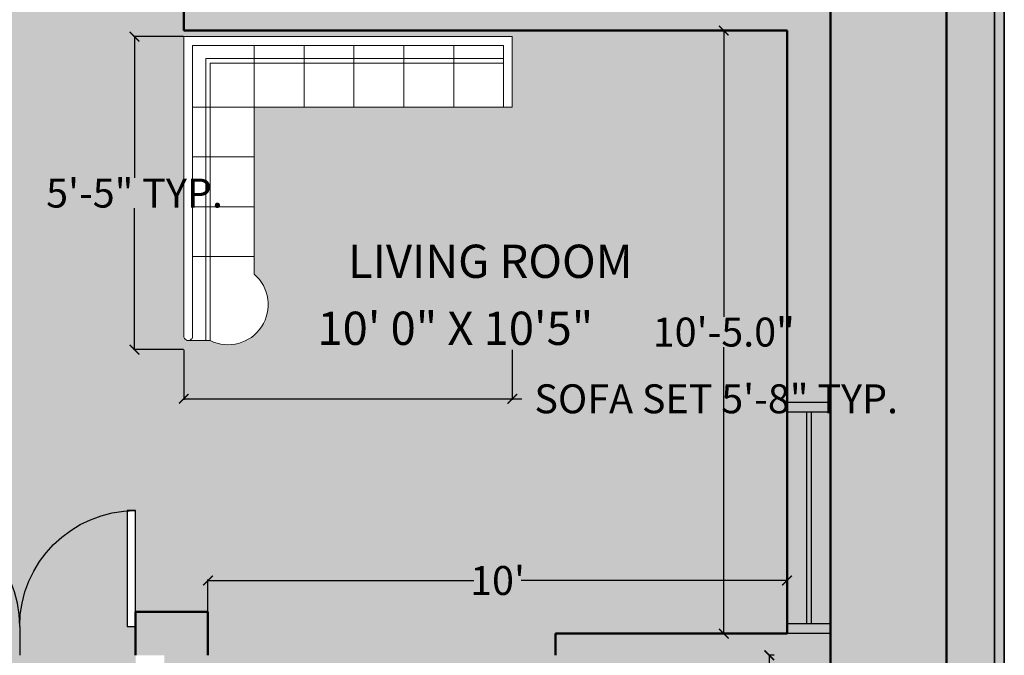
# Model space of a CAD drawing. Units: inches. Extents: x 528 to 2620, y -1066 to 798.
# Tile 4 of 41: x 740 to 944, y 391 to 523. Entities that reach past the tile are written whole.
import ezdxf

# ---------------------------------------------------------------- set-up
doc = ezdxf.new("R2010")
doc.units = ezdxf.units.IN
doc.header["$MEASUREMENT"] = 0
for name, color, linetype, lineweight in [('A-ANNO-DIMS', 2, 'Continuous', 18), ('A-AREA-IDEN', 7, 'Continuous', 18), ('A-Door', 2, 'Continuous', 25), ('A-FURN', 30, 'Continuous', 18), ('A-GLAZ', 3, 'Continuous', 25), ('A-WALL', 7, 'Continuous', 50), ('A-WALL-PATT', 8, 'Continuous', 13), ('C-PROP', 5, 'Continuous', 35)]:
    doc.layers.add(name, color=color, linetype=linetype, lineweight=lineweight)
doc.styles.get("Standard").update_dxf_attribs({"font": 'arial.ttf'})
doc.dimstyles.get("Standard").update_dxf_attribs({"dimtxt": 6, "dimasz": 2, "dimexe": 0.18, "dimexo": 0.0625, "dimgap": 0.09, "dimtad": 0, "dimtih": 1, "dimtoh": 1, "dimdec": 1, "dimzin": 0, "dimdsep": 46, "dimlunit": 3, "dimtxsty": 'Standard', "dimblk": 'ARCHTICK', "dimcen": 0.09, "dimadec": 0, "dimazin": 0, "dimtfac": 1, "dimtdec": 1, "dimtofl": 0, "dimtmove": 0, "dimatfit": 3, "dimfxl": 1, "dimtolj": 1, "dimtzin": 0, "dimarcsym": 0})

# ---------------------------------------------------------------- blocks, each defined once
blk = doc.blocks.new('*U3')
for p, q in [((0, 0), (0, -6)), ((24, 0), (24, -6))]:
    blk.add_line(p, q)
blk.add_lwpolyline([(0, 0), (0, 24), (1.75, 24), (1.75, 0)], close=True)
blk.add_arc((0, 0), 24, 0, 90)
blk = doc.blocks.new('QU')
at = {"color": 0}
for p, q in [((-0.8, -2.5), (-0.8, 1.233)), ((-0.8, 1.233), (0, 1.233)), ((0, 1.233), (0, -2.4)), ((-0.7, -2.4), (-0.7, 1.133)), ((-0.7, 1.133), (0, 1.133)), ((-0.55, -2.25), (-0.55, 1.133)), ((-0.5, -2.2), (-0.5, 1.133)), ((-0.7, 0.567), (0, 0.567)), ((-0.7, 0), (0, 0)), ((-0.7, -0.567), (0, -0.567)), ((-0.7, -1.133), (0, -1.133)), ((-0.7, -1.7), (1.133, -1.7)), ((-0.133, -1.7), (1.7, -1.7)), ((0.567, -1.7), (0.567, -2.4)), ((1.133, -1.7), (1.133, -2.4)), ((1.133, -1.7), (1.133, -2.4)), ((1.7, -1.7), (1.9, -1.7)), ((1.7, -1.7), (1.7, -2.4)), ((2.655, -2.2), (-0.5, -2.2)), ((2.655, -2.45), (2.655, -2.2)), ((2.655, -2.25), (-0.55, -2.25)), ((2.605, -2.4), (-0.7, -2.4)), ((2.605, -2.5), (-0.8, -2.5))]:
    blk.add_line(p, q, dxfattribs=at)
for centre, radius, start, end in [((2.247, -1.997), 0.456, 333.5922, 139.3979), ((2.605, -2.45), 0.05, 270, 90)]:
    blk.add_arc(centre, radius, start, end, dxfattribs=at)
blk = doc.blocks.new('_ArchTick')
at = {"color": 0, "linetype": 'ByBlock', "const_width": 0.15}
blk.add_lwpolyline([(-0.5, -0.5), (0.5, 0.5)], dxfattribs=at)
blk = doc.blocks.new('*D33')
at = {"layer": 'A-ANNO-DIMS', "color": 0, "lineweight": -2, "transparency": 16777216}
for p, q in [((896.35, 391.42), (895.19, 391.42)), ((895.37, 391.42), (895.37, 337.83)), ((895.37, 277.92), (895.37, 331.52)), ((896.35, 277.92), (895.19, 277.92))]:
    blk.add_line(p, q, dxfattribs=at)
at = {"layer": 'Defpoints', "color": 0, "transparency": 16777216}
for p in [(896.41, 391.42), (895.37, 277.92), (896.41, 277.92)]:
    blk.add_point(p, dxfattribs=at)
at = {"layer": 'A-ANNO-DIMS', "color": 0, "lineweight": -2, "transparency": 16777216, "xscale": 2, "yscale": 2, "zscale": 2}
for p, rotation in [((895.37, 391.42), 90), ((895.37, 277.92), 270)]:
    blk.add_blockref('_ArchTick', p, dxfattribs=dict(at, rotation=rotation))
at = {"layer": 'A-ANNO-DIMS', "color": 0, "transparency": 16777216, "insert": (895.37, 334.67), "char_height": 6, "attachment_point": 5}
blk.add_mtext('\\A1;9\'-5.5"', dxfattribs=at)
blk = doc.blocks.new('*D35')
at = {"layer": 'A-ANNO-DIMS', "color": 0, "lineweight": -2, "transparency": 16777216}
for p, q in [((891.94, 520.92), (885.76, 520.92)), ((885.94, 520.92), (885.94, 461.58)), ((885.94, 395.92), (885.94, 455.27)), ((891.94, 395.92), (885.76, 395.92))]:
    blk.add_line(p, q, dxfattribs=at)
at = {"layer": 'Defpoints', "color": 0, "transparency": 16777216}
for p in [(892, 520.92), (885.94, 395.92), (892, 395.92)]:
    blk.add_point(p, dxfattribs=at)
at = {"layer": 'A-ANNO-DIMS', "color": 0, "lineweight": -2, "transparency": 16777216, "xscale": 2, "yscale": 2, "zscale": 2}
for p, rotation in [((885.94, 520.92), 90), ((885.94, 395.92), 270)]:
    blk.add_blockref('_ArchTick', p, dxfattribs=dict(at, rotation=rotation))
at = {"layer": 'A-ANNO-DIMS', "color": 0, "transparency": 16777216, "insert": (885.94, 458.42), "char_height": 6, "attachment_point": 5}
blk.add_mtext('\\A1;10\'-5.0"', dxfattribs=at)
blk = doc.blocks.new('*D36')
at = {"layer": 'A-ANNO-DIMS', "color": 0, "lineweight": -2, "transparency": 16777216}
for p, q in [((779.06, 400.48), (779.06, 407.11)), ((779.06, 406.93), (834.16, 406.93)), ((899.06, 406.93), (843.96, 406.93)), ((899.06, 400.48), (899.06, 407.11))]:
    blk.add_line(p, q, dxfattribs=at)
at = {"layer": 'Defpoints', "color": 0, "transparency": 16777216}
for p in [(899.06, 406.93), (779.06, 400.42), (899.06, 400.42)]:
    blk.add_point(p, dxfattribs=at)
at = {"layer": 'A-ANNO-DIMS', "color": 0, "lineweight": -2, "transparency": 16777216, "xscale": 2, "yscale": 2, "zscale": 2, "rotation": 180}
blk.add_blockref('_ArchTick', (779.06, 406.93), dxfattribs=at)
at = {"layer": 'A-ANNO-DIMS', "color": 0, "lineweight": -2, "transparency": 16777216, "xscale": 2, "yscale": 2, "zscale": 2}
blk.add_blockref('_ArchTick', (899.06, 406.93), dxfattribs=at)
at = {"layer": 'A-ANNO-DIMS', "color": 0, "transparency": 16777216, "insert": (839.06, 406.93), "char_height": 6, "attachment_point": 5}
blk.add_mtext("\\A1;10'", dxfattribs=at)
blk = doc.blocks.new('WIN-1200')
for p, q in [((677.56, 718.92), (725.56, 718.92)), ((677.56, 709.92), (677.56, 718.92)), ((679.56, 709.92), (679.56, 718.92)), ((723.56, 718.92), (723.56, 709.92)), ((725.56, 718.92), (725.56, 709.92)), ((679.56, 714.92), (723.56, 714.92)), ((679.56, 713.92), (723.56, 713.92)), ((725.56, 709.92), (677.56, 709.92))]:
    blk.add_line(p, q)
blk = doc.blocks.new('*D44')
at = {"layer": 'A-ANNO-DIMS', "color": 0, "lineweight": -2, "transparency": 16777216}
for p, q in [((774.06, 454.73), (774.06, 444.41)), ((842.12, 454.73), (842.12, 444.41)), ((774.06, 444.59), (842.12, 444.59)), ((842.12, 444.59), (844.12, 444.59))]:
    blk.add_line(p, q, dxfattribs=at)
at = {"layer": 'Defpoints', "color": 0, "transparency": 16777216}
for p in [(774.06, 454.8), (842.12, 454.8), (842.12, 444.59)]:
    blk.add_point(p, dxfattribs=at)
at = {"layer": 'A-ANNO-DIMS', "color": 0, "lineweight": -2, "transparency": 16777216, "xscale": 2, "yscale": 2, "zscale": 2, "rotation": 180}
blk.add_blockref('_ArchTick', (774.06, 444.59), dxfattribs=at)
at = {"layer": 'A-ANNO-DIMS', "color": 0, "lineweight": -2, "transparency": 16777216, "xscale": 2, "yscale": 2, "zscale": 2}
blk.add_blockref('_ArchTick', (842.12, 444.59), dxfattribs=at)
at = {"layer": 'A-ANNO-DIMS', "color": 0, "transparency": 16777216, "insert": (884.37, 444.59), "char_height": 6, "attachment_point": 5}
blk.add_mtext('\\A1;SOFA SET 5\'-8" TYP.', dxfattribs=at)
blk = doc.blocks.new('*D45')
at = {"layer": 'A-ANNO-DIMS', "color": 0, "lineweight": -2, "transparency": 16777216}
for p, q in [((774, 519.66), (763.67, 519.66)), ((763.85, 519.66), (763.85, 490.37)), ((763.85, 454.8), (763.85, 484.09)), ((774, 454.8), (763.67, 454.8))]:
    blk.add_line(p, q, dxfattribs=at)
at = {"layer": 'Defpoints', "color": 0, "transparency": 16777216}
for p in [(774.06, 519.66), (763.85, 454.8), (774.06, 454.8)]:
    blk.add_point(p, dxfattribs=at)
at = {"layer": 'A-ANNO-DIMS', "color": 0, "lineweight": -2, "transparency": 16777216, "xscale": 2, "yscale": 2, "zscale": 2}
for p, rotation in [((763.85, 519.66), 90), ((763.85, 454.8), 270)]:
    blk.add_blockref('_ArchTick', p, dxfattribs=dict(at, rotation=rotation))
at = {"layer": 'A-ANNO-DIMS', "color": 0, "transparency": 16777216, "insert": (763.85, 487.23), "char_height": 6, "attachment_point": 5}
blk.add_mtext('\\A1;5\'-5" TYP.', dxfattribs=at)

msp = doc.modelspace()

# ---------------------------------------------------------------- hatches: boundary and pattern name
at = {"layer": 'A-WALL-PATT', "transparency": 33554687}
h = msp.add_hatch(color=256, dxfattribs=at)
h.dxf.hatch_style = 1
h.paths.add_polyline_path([(944.06, 753.92), (584.06, 753.92), (584.06, 208.92), (608.06, 208.92), (608.06, 210.92), (586.06, 210.92), (586.06, 751.92), (942.06, 751.92), (942.06, 210.92), (728.06, 210.92), (728.06, 208.92), (944.06, 208.92)])
h = msp.add_hatch(color=256, dxfattribs=at)
h.dxf.hatch_style = 1
h.paths.add_polyline_path([(942.06, 751.92), (586.06, 751.92), (586.06, 210.92), (608.06, 210.92), (608.06, 220.92), (596.06, 220.92), (596.06, 741.92), (932.06, 741.92), (932.06, 220.92), (770.06, 220.92), (728.06, 220.92), (728.06, 210.92), (942.06, 210.92)])
at = {"layer": 'A-WALL-PATT', "transparency": 33554475}
h = msp.add_hatch(color=256, dxfattribs=at)
h.dxf.hatch_style = 1
h.paths.add_polyline_path([(620.06, 718.92), (908.06, 718.92), (908.06, 268.92), (770.06, 268.92), (770.06, 220.92), (932.06, 220.92), (932.06, 741.92), (596.06, 741.92), (596.06, 391.42), (620.06, 391.42)])
at = {"layer": 'A-WALL-PATT', "transparency": 33554687}
h = msp.add_hatch(color=256, dxfattribs=at)
h.dxf.hatch_style = 1
h.paths.add_polyline_path([(861.06, 273.92), (817.06, 273.92), (817.06, 272.92), (861.06, 272.92)])
h.paths.add_polyline_path([(817.06, 277.92), (815.06, 277.92), (815.06, 268.92), (817.06, 268.92)])
h.paths.add_polyline_path([(908.06, 397.92), (899.06, 397.92), (899.06, 395.92), (908.06, 395.92)])
h.paths.add_polyline_path([(908.06, 443.92), (899.06, 443.92), (899.06, 441.92), (908.06, 441.92)])
h.paths.add_polyline_path([(904.06, 441.92), (903.06, 441.92), (903.06, 397.92), (904.06, 397.92)])
h.paths.add_polyline_path([(625.06, 561.42), (624.06, 561.42), (624.06, 537.42), (625.06, 537.42)])
h.paths.add_polyline_path([(648.75, 334.44), (720.04, 334.44), (720.04, 345), (648.75, 345)], flags=9)
h.paths.add_polyline_path([(819.73, 323.15), (880.33, 323.15), (880.33, 333.71), (819.73, 333.71)], flags=9)
h.paths.add_polyline_path([(779.9, 680.61), (821.76, 680.61), (821.76, 691.17), (779.9, 691.17)], flags=9)
h.paths.add_polyline_path([(779.88, 692.36), (817.14, 692.36), (817.14, 703.06), (779.88, 703.06)], flags=9)
h.paths.add_polyline_path([(799.99, 453.88), (860.59, 453.88), (860.59, 464.44), (799.99, 464.44)], flags=9)
h.paths.add_polyline_path([(650.87, 539.4), (708.78, 539.4), (708.78, 549.95), (650.87, 549.95)], flags=9)
h.paths.add_polyline_path([(788.5, 612.01), (849.1, 612.01), (849.1, 622.56), (788.5, 622.56)], flags=9)
h.paths.add_polyline_path([(639.54, 648.31), (700.13, 648.31), (700.13, 658.87), (639.54, 658.87)], flags=9)
h.paths.add_polyline_path([(648.91, 346.09), (747.71, 346.09), (747.71, 356.78), (648.91, 356.78)], flags=9)
h.paths.add_polyline_path([(676.86, 450.66), (746.74, 450.66), (746.74, 461.36), (676.86, 461.36)], flags=9)
h.paths.add_polyline_path([(819.71, 334.95), (865.53, 334.95), (865.53, 345.64), (819.71, 345.64)], flags=9)
h.paths.add_polyline_path([(806.3, 467.75), (874.05, 467.75), (874.05, 478.44), (806.3, 478.44)], flags=9)
h.paths.add_polyline_path([(653.23, 552.28), (690.5, 552.28), (690.5, 562.98), (653.23, 562.98)], flags=9)
h.paths.add_polyline_path([(789.9, 623.41), (843.21, 623.41), (843.21, 634.1), (789.9, 634.1)], flags=9)
h.paths.add_polyline_path([(639.77, 662.1), (693.08, 662.1), (693.08, 672.8), (639.77, 672.8)], flags=9)
h.paths.add_polyline_path([(801.59, 242.91), (846.33, 242.91), (846.33, 253.6), (801.59, 253.6)], flags=9)
h.paths.add_polyline_path([(925.36, 593.98), (925.36, 674.06), (914.67, 674.06), (914.67, 593.98)], flags=9)
h.paths.add_polyline_path([(612.56, 593.98), (612.56, 674.06), (601.87, 674.06), (601.87, 593.98)], flags=9)
h.paths.add_polyline_path([(723.31, 726.56), (803.39, 726.56), (803.39, 737.25), (723.31, 737.25)], flags=9)
at = {"layer": 'A-WALL-PATT', "transparency": 33554521}
h = msp.add_hatch(color=256, dxfattribs=at)
h.dxf.hatch_style = 1
h.paths.add_polyline_path([(629.06, 709.92), (677.56, 709.92), (677.56, 718.92), (620.06, 718.92), (620.06, 667.92), (629.06, 667.92)])
h.paths.add_polyline_path([(790.56, 718.92), (725.56, 718.92), (725.56, 709.92), (774.06, 709.92), (774.06, 577.92), (768.48, 577.92), (768.56, 573.42), (774.06, 573.42), (774.06, 567.42), (778.56, 567.42), (778.56, 669.42), (831.06, 669.42), (831.06, 675.92), (826.56, 675.92), (826.56, 673.92), (778.56, 673.92), (778.56, 709.92), (790.56, 709.92)])
h.paths.add_polyline_path([(908.06, 718.92), (879.06, 718.92), (879.06, 709.92), (899.06, 709.92), (899.06, 641.67), (908.06, 641.67)])
h.paths.add_polyline_path([(629.06, 619.92), (620.06, 619.92), (620.06, 561.42), (629.06, 561.42), (629.06, 573.42), (724.06, 573.42), (724.06, 569.42), (728.56, 569.42), (728.56, 577.92), (629.06, 577.92)])
h.paths.add_polyline_path([(779.06, 391.42), (779.06, 400.42), (770.06, 400.42), (764.06, 400.42), (764.06, 397.42), (764.06, 391.42), (770.06, 391.42), (770.06, 268.92), (815.06, 268.92), (815.06, 277.92), (779.06, 277.92), (779.06, 359.77)])
h.paths.add_polyline_path([(908.06, 395.92), (899.06, 395.92), (851.06, 395.92), (851.06, 391.42), (899.06, 391.42), (899.06, 277.92), (863.06, 277.92), (863.06, 268.92), (908.06, 268.92)])
h.paths.add_polyline_path([(908.06, 593.67), (899.06, 593.67), (899.06, 525.42), (778.56, 525.42), (778.56, 527.17), (774.06, 527.17), (774.06, 520.92), (899.06, 520.92), (899.06, 443.92), (908.06, 443.92)])
h.paths.add_polyline_path([(629.06, 520.92), (728.56, 520.92), (728.56, 545.42), (724.06, 545.42), (724.06, 525.42), (629.06, 525.42), (629.06, 537.42), (620.06, 537.42), (620.06, 484.67), (629.06, 484.67)])
h.paths.add_polyline_path([(629.06, 436.67), (620.06, 436.67), (620.06, 391.42), (648.56, 391.42), (648.56, 400.42), (629.06, 400.42)])
h.paths.add_polyline_path([(716.06, 397.42), (716.06, 400.42), (696.56, 400.42), (696.56, 391.42), (716.06, 391.42)])
at = {"layer": 'A-WALL-PATT', "transparency": 33554681}
h = msp.add_hatch(color=256, dxfattribs=at)
h.dxf.hatch_style = 1
h.paths.add_polyline_path([(629.06, 665.92), (625.06, 665.92), (625.06, 621.92), (629.06, 621.92)])
h.paths.add_polyline_path([(624.06, 665.92), (620.06, 665.92), (620.06, 621.92), (624.06, 621.92)])
h.paths.add_polyline_path([(723.56, 713.92), (679.56, 713.92), (679.56, 709.92), (723.56, 709.92)])
h.paths.add_polyline_path([(723.56, 718.92), (679.56, 718.92), (679.56, 714.92), (723.56, 714.92)])
h.paths.add_polyline_path([(814.56, 713.92), (790.56, 713.92), (790.56, 709.92), (814.56, 709.92)])
h.paths.add_polyline_path([(814.56, 718.92), (790.56, 718.92), (790.56, 714.92), (814.56, 714.92)])
h.paths.add_polyline_path([(877.06, 713.92), (833.06, 713.92), (833.06, 709.92), (877.06, 709.92)])
h.paths.add_polyline_path([(877.06, 718.92), (833.06, 718.92), (833.06, 714.92), (877.06, 714.92)])
h.paths.add_polyline_path([(908.06, 639.67), (904.06, 639.67), (904.06, 595.67), (908.06, 595.67)])
h.paths.add_polyline_path([(903.06, 639.67), (899.06, 639.67), (899.06, 595.67), (903.06, 595.67)])
h.paths.add_polyline_path([(908.06, 441.92), (904.06, 441.92), (904.06, 397.92), (908.06, 397.92)])
h.paths.add_polyline_path([(903.06, 441.92), (899.06, 441.92), (899.06, 397.92), (903.06, 397.92)])
h.paths.add_polyline_path([(861.06, 272.92), (817.06, 272.92), (817.06, 268.92), (861.06, 268.92)])
h.paths.add_polyline_path([(861.06, 277.92), (817.06, 277.92), (817.06, 273.92), (861.06, 273.92)])
h.paths.add_polyline_path([(694.56, 395.42), (650.56, 395.42), (650.56, 391.42), (694.56, 391.42)])
h.paths.add_polyline_path([(694.56, 400.42), (650.56, 400.42), (650.56, 396.42), (694.56, 396.42)])
h.paths.add_polyline_path([(629.06, 482.67), (625.06, 482.67), (625.06, 438.67), (629.06, 438.67)])
h.paths.add_polyline_path([(624.06, 482.67), (620.06, 482.67), (620.06, 438.67), (624.06, 438.67)])
h.paths.add_polyline_path([(629.06, 561.42), (625.06, 561.42), (625.06, 537.42), (629.06, 537.42)])
h.paths.add_polyline_path([(624.06, 561.42), (620.06, 561.42), (620.06, 537.42), (624.06, 537.42)])
at = {"layer": 'A-WALL-PATT', "transparency": 33554590}
h = msp.add_hatch(color=256, dxfattribs=at)
h.dxf.hatch_style = 1
h.paths.add_polyline_path([(774.06, 709.92), (629.06, 709.92), (629.06, 577.92), (728.56, 577.92), (728.56, 579.42), (728.56, 619.42), (730.31, 619.42), (730.31, 619.38, -0.401453), (768.56, 579.42), (768.56, 577.92), (774.06, 577.92)])
h.paths.add_polyline_path([(723.9, 686.06), (723.97, 686.06), (723.83, 686.13)], flags=0)
h.paths.add_polyline_path([(722.79, 642.7), (722.89, 642.76), (722.89, 684.99), (722.65, 685.24), (722.65, 685.82), (723.08, 686.26), (723.53, 686.26), (723.97, 686.06), (724.74, 686.13), (770.7, 686.13), (770.78, 686.14), (771.13, 686.27), (771.69, 686.09), (771.94, 685.48), (771.67, 684.9), (771.58, 684.87), (771.58, 642.78), (771.88, 642.51), (771.88, 641.92), (771.51, 641.46), (770.85, 641.46), (770.4, 641.83), (770.4, 641.55), (724.74, 641.55), (723.99, 641.7), (723.44, 641.41), (722.88, 641.59), (722.6, 642.14)], flags=16)
h.paths.add_polyline_path([(723.99, 641.7), (723.99, 641.71), (723.99, 641.7)], flags=0)
h.paths.add_polyline_path([(722.89, 642.73), (722.89, 684.99), (722.65, 685.24), (722.65, 685.82), (723.08, 686.26), (723.29, 686.26), (722.99, 686.17), (722.79, 685.97), (722.65, 685.68), (722.65, 685.43), (722.75, 685.14), (722.94, 684.94), (723.24, 684.81), (723.48, 684.81), (723.78, 684.9), (723.98, 685.1), (724.17, 685.49), (724.12, 685.64), (724.12, 685.25), (723.63, 684.75), (723.63, 642.96), (724.12, 642.51), (724.12, 641.89), (723.66, 641.46), (723.08, 641.46), (722.65, 641.9), (722.65, 642.48)], flags=0)
h.paths.add_polyline_path([(722.65, 642.29), (722.65, 642.04), (722.79, 641.75), (723.08, 641.46), (723.29, 641.46), (722.88, 641.59), (722.6, 642.14)], flags=0)
h.paths.add_polyline_path([(770.75, 686.13), (770.58, 686.13), (770.55, 686.06)], flags=0)
h.paths.add_polyline_path([(743.3, 645.29), (753.23, 659.4), (748.69, 663.75), (753.23, 668.54), (743.3, 682.46), (743.79, 682.59), (744.14, 682.68), (744.53, 682.93), (744.63, 683.08), (745.02, 683.33), (744.53, 684.07), (744.78, 684.16), (744.87, 684.31), (745.51, 684.4), (746.08, 684.65), (746.47, 684.65), (746.82, 684.81), (747.46, 685.03), (747.71, 685.14), (748.2, 685.28), (748.39, 685.52), (748.86, 685.52), (749.99, 686.13), (753.49, 676.03), (757.38, 680.15), (757.79, 679.76), (758.04, 680.65), (758.29, 681.23), (758.29, 682.05), (758.02, 682.59), (757.87, 683.17), (757.82, 683.78), (758.39, 684.07), (758.98, 684.2), (759.62, 684.16), (760.21, 683.96), (760.75, 683.67), (761.86, 683.67), (762.4, 683.96), (762.99, 684.11), (763.63, 684.11), (764.2, 683.96), (764.74, 683.67), (766.12, 683.67), (766.66, 683.96), (767.25, 684.16), (767.87, 684.2), (768.46, 684.07), (769.05, 683.78), (769, 683.17), (768.85, 682.59), (768.55, 682.05), (768.55, 681.23), (768.8, 680.65), (769.09, 679.75), (768.95, 678.83), (768.8, 678.23), (768.55, 677.65), (768.55, 676.82), (768.8, 676.24), (769.09, 675.34), (768.95, 674.42), (768.8, 673.82), (768.55, 673.28), (768.55, 672.41), (768.8, 671.87), (769, 671.29), (769.05, 670.64), (768.95, 670.02), (768.8, 669.41), (768.55, 668.87), (768.55, 668), (768.97, 667.24), (769.05, 666.28), (769.05, 665.56), (768.46, 665.32), (767.87, 665.16), (767.25, 665.16), (766.66, 665.36), (766.12, 665.7), (764.74, 665.7), (763.94, 665.2), (762.99, 665.2), (762.4, 665.36), (761.86, 665.7), (761, 665.7), (762.7, 664.09), (760.74, 662.03), (761.86, 662.03), (762.4, 662.32), (763.34, 662.55), (764.25, 662.32), (764.79, 662.03), (766.12, 662.03), (766.66, 662.32), (767.25, 662.52), (767.87, 662.56), (768.51, 662.43), (769.05, 662.12), (769.05, 661.4), (769.05, 660.8), (768.85, 660.21), (768.55, 659.68), (768.55, 658.85), (768.85, 658.27), (769, 657.66), (769.07, 656.75), (768.85, 655.85), (768.55, 655.27), (768.55, 654.44), (768.85, 653.86), (769.07, 652.96), (769, 652.05), (768.85, 651.44), (768.55, 650.91), (768.55, 650.03), (768.85, 649.5), (769, 648.91), (769.05, 648.26), (769, 647.64), (768.85, 647.03), (768.55, 646.5), (768.55, 645.62), (768.85, 645.09), (769.05, 644.55), (769.05, 643.9), (768.51, 643.65), (767.87, 643.52), (767.25, 643.52), (766.66, 643.72), (766.12, 644.06), (764.79, 644.06), (764.25, 643.72), (763.34, 643.49), (762.4, 643.72), (761.86, 644.06), (760.8, 644.06), (760.26, 643.72), (759.67, 643.52), (759.03, 643.52), (758.39, 643.65), (757.87, 643.9), (757.87, 644.55), (758.04, 645.09), (758.34, 645.62), (758.34, 646.5), (758.04, 647.03), (757.92, 647.64), (757.87, 648.06), (757.38, 647.59), (753.42, 651.77), (749.99, 641.62), (749.5, 641.71), (749.35, 641.95), (748.54, 642.45), (747.31, 642.94), (746.65, 642.94), (746.33, 643.18), (745.51, 643.57), (744.53, 643.65), (745.01, 644.4), (744.63, 644.64), (744.14, 644.89), (743.79, 645.13)], flags=0)
h.paths.add_polyline_path([(755.66, 654.93), (756.54, 654.69), (757.53, 654.33), (756.64, 654.58)], flags=0)
h.paths.add_polyline_path([(758.34, 649.2), (758.34, 648.71), (758.59, 644.3), (758.59, 648.8)], flags=0)
h.paths.add_polyline_path([(758.34, 649.29), (758.09, 649.7), (758.36, 649.17)], flags=0)
h.paths.add_polyline_path([(755.66, 672.79), (756.49, 673.04), (757.36, 673.35), (757.35, 673.36), (756.64, 673.15)], flags=0)
h.paths.add_polyline_path([(760.26, 639.64), (771.41, 639.64), (771.41, 624.04), (760.26, 624.04)], flags=16)
h.paths.add_polyline_path([(761.38, 638.53), (770.29, 638.53), (770.29, 625.15), (761.38, 625.15)], flags=0)
edge = h.paths.add_edge_path(flags=0)
edge.add_ellipse((765.84, 631.84), major_axis=(-2.24, 2.24), ratio=1, start_angle=-45, end_angle=45, ccw=False)
edge.add_ellipse((765.84, 631.84), major_axis=(-2.24, 2.24), ratio=1, start_angle=-135, end_angle=-45, ccw=False)
edge.add_ellipse((765.84, 631.84), major_axis=(-2.24, 2.24), ratio=1, start_angle=135, end_angle=-135, ccw=False)
edge.add_ellipse((765.84, 631.84), major_axis=(-2.24, 2.24), ratio=1, start_angle=45, end_angle=135, ccw=False)
h.paths.add_polyline_path([(758.59, 683.42), (758.59, 678.92), (758.37, 678.58), (758.34, 678.43), (758.09, 678.05), (758.34, 678.52), (758.34, 679.01)], flags=0)
h.paths.add_polyline_path([(760.26, 688.04), (760.26, 703.64), (771.41, 703.64), (771.41, 688.04)], flags=16)
h.paths.add_polyline_path([(770.4, 685.39), (770.4, 685.85), (770.85, 686.22), (771.51, 686.22), (771.88, 685.76), (771.88, 685.17), (771.58, 684.9), (771.58, 642.78), (771.88, 642.51), (771.88, 641.92), (771.51, 641.46), (770.85, 641.46), (770.4, 641.83), (770.4, 642.29)], flags=0)
h.paths.add_polyline_path([(770.53, 642.68), (771.05, 643.01), (771.67, 642.77), (771.94, 642.2), (771.69, 641.59), (771.13, 641.41), (770.55, 641.62), (770.35, 642.13)], flags=16)
h.paths.add_polyline_path([(761.38, 689.15), (761.38, 702.53), (770.29, 702.53), (770.29, 689.15)], flags=0)
edge = h.paths.add_edge_path(flags=0)
edge.add_ellipse((765.84, 695.84), major_axis=(2.24, 2.24), ratio=1, start_angle=405, end_angle=495, ccw=False)
edge.add_ellipse((765.84, 695.84), major_axis=(2.24, 2.24), ratio=1, start_angle=675, end_angle=765, ccw=False)
edge.add_ellipse((765.84, 695.84), major_axis=(2.24, 2.24), ratio=1, start_angle=585, end_angle=675, ccw=False)
edge.add_ellipse((765.84, 695.84), major_axis=(2.24, 2.24), ratio=1, start_angle=495, end_angle=585, ccw=False)
h.paths.add_polyline_path([(770.7, 684.9), (770.94, 684.74), (771.41, 684.74), (771.73, 685.03), (771.88, 685.34), (771.88, 685.64), (771.69, 686.09), (771.58, 686.13), (771.88, 685.76), (771.88, 685.17), (771.41, 684.74), (770.85, 684.74)], flags=0)
h.paths.add_polyline_path([(899.06, 709.92), (831.06, 709.92), (831.06, 699.92), (829.81, 699.92), (829.81, 675.92), (831.06, 675.92), (831.06, 669.42), (778.56, 669.42), (778.56, 567.17), (780.06, 567.17), (820.06, 567.17), (820.06, 565.42), (820.02, 565.42, -0.401453), (780.06, 527.17), (778.56, 527.17), (778.56, 525.42), (899.06, 525.42)])
h.paths.add_polyline_path([(849.2, 636.01), (849.27, 636.02), (849.13, 636.08)], flags=0)
h.paths.add_polyline_path([(848.19, 634.95), (847.95, 635.2), (847.95, 635.78), (848.38, 636.22), (848.83, 636.22), (849.27, 636.02), (850.04, 636.08), (896, 636.08), (896.08, 636.1), (896.43, 636.22), (896.99, 636.05), (897.24, 635.43), (896.97, 634.86), (896.88, 634.83), (896.88, 592.74), (897.18, 592.47), (897.18, 591.88), (896.81, 591.42), (896.15, 591.42), (895.7, 591.79), (895.7, 591.51), (850.04, 591.51), (849.29, 591.66), (848.74, 591.37), (848.18, 591.54), (847.9, 592.1), (848.09, 592.65), (848.19, 592.71)], flags=16)
h.paths.add_polyline_path([(849.29, 591.66), (849.29, 591.66), (849.29, 591.66)], flags=16)
h.paths.add_polyline_path([(848.19, 634.95), (847.95, 635.2), (847.95, 635.78), (848.38, 636.22), (848.59, 636.22), (848.29, 636.13), (848.09, 635.93), (847.95, 635.64), (847.95, 635.39), (848.05, 635.1), (848.24, 634.9), (848.54, 634.76), (848.78, 634.76), (849.08, 634.85), (849.28, 635.05), (849.47, 635.44), (849.42, 635.59), (849.42, 635.21), (848.93, 634.7), (848.93, 592.92), (849.42, 592.47), (849.42, 591.84), (848.96, 591.42), (848.38, 591.42), (847.95, 591.86), (847.95, 592.44), (848.19, 592.69)], flags=0)
h.paths.add_polyline_path([(847.95, 592.25), (847.95, 592), (848.09, 591.71), (848.38, 591.42), (848.59, 591.42), (848.18, 591.54), (847.9, 592.1)], flags=16)
h.paths.add_polyline_path([(896.05, 636.08), (895.88, 636.08), (895.85, 636.01)], flags=0)
h.paths.add_polyline_path([(868.6, 632.41), (869.09, 632.55), (869.44, 632.64), (869.83, 632.88), (869.93, 633.04), (870.32, 633.28), (869.83, 634.02), (870.08, 634.11), (870.17, 634.27), (870.81, 634.36), (871.38, 634.61), (871.77, 634.61), (872.12, 634.76), (872.76, 634.99), (873.01, 635.1), (873.5, 635.23), (873.69, 635.48), (874.16, 635.48), (875.29, 636.08), (878.79, 625.99), (882.68, 630.11), (883.09, 629.71), (883.34, 630.6), (883.59, 631.18), (883.59, 632.01), (883.32, 632.55), (883.17, 633.13), (883.12, 633.73), (883.69, 634.02), (884.28, 634.16), (884.92, 634.11), (885.51, 633.91), (886.05, 633.62), (887.16, 633.62), (887.7, 633.91), (888.29, 634.07), (888.93, 634.07), (889.5, 633.91), (890.04, 633.62), (891.42, 633.62), (891.96, 633.91), (892.55, 634.11), (893.17, 634.16), (893.76, 634.02), (894.35, 633.73), (894.3, 633.13), (894.15, 632.55), (893.85, 632.01), (893.85, 631.18), (894.1, 630.6), (894.39, 629.71), (894.25, 628.79), (894.1, 628.18), (893.85, 627.6), (893.85, 626.77), (894.1, 626.19), (894.39, 625.3), (894.25, 624.38), (894.1, 623.78), (893.85, 623.24), (893.85, 622.37), (894.1, 621.83), (894.3, 621.25), (894.35, 620.6), (894.25, 619.97), (894.1, 619.37), (893.85, 618.83), (893.85, 617.96), (894.27, 617.2), (894.35, 616.23), (894.35, 615.52), (893.76, 615.27), (893.17, 615.12), (892.55, 615.12), (891.96, 615.32), (891.42, 615.65), (890.04, 615.65), (889.25, 615.16), (888.29, 615.16), (887.7, 615.32), (887.16, 615.65), (886.31, 615.65), (888, 614.04), (886.04, 611.98), (887.16, 611.98), (887.7, 612.27), (888.64, 612.5), (889.55, 612.27), (890.09, 611.98), (891.42, 611.98), (891.96, 612.27), (892.55, 612.48), (893.17, 612.52), (893.81, 612.39), (894.35, 612.07), (894.35, 611.36), (894.35, 610.75), (894.15, 610.17), (893.85, 609.63), (893.85, 608.81), (894.15, 608.22), (894.3, 607.62), (894.37, 606.7), (894.15, 605.81), (893.85, 605.22), (893.85, 604.4), (894.15, 603.81), (894.37, 602.92), (894.3, 602), (894.15, 601.4), (893.85, 600.86), (893.85, 599.99), (894.15, 599.45), (894.3, 598.87), (894.35, 598.22), (894.3, 597.59), (894.15, 596.99), (893.85, 596.45), (893.85, 595.58), (894.15, 595.04), (894.35, 594.51), (894.35, 593.86), (893.81, 593.61), (893.17, 593.48), (892.55, 593.48), (891.96, 593.68), (891.42, 594.01), (890.09, 594.01), (889.55, 593.68), (888.64, 593.45), (887.7, 593.68), (887.16, 594.01), (886.1, 594.01), (885.56, 593.68), (884.97, 593.48), (884.33, 593.48), (883.69, 593.61), (883.17, 593.86), (883.17, 594.51), (883.34, 595.04), (883.64, 595.58), (883.64, 596.45), (883.34, 596.99), (883.22, 597.59), (883.17, 598.01), (882.68, 597.55), (878.72, 601.73), (875.29, 591.57), (874.8, 591.66), (874.65, 591.91), (873.84, 592.4), (872.61, 592.89), (871.95, 592.89), (871.63, 593.14), (870.81, 593.52), (869.83, 593.61), (870.31, 594.36), (869.93, 594.6), (869.44, 594.84), (869.09, 595.09), (868.6, 595.24), (878.53, 609.35), (873.99, 613.71), (878.53, 618.49)], flags=0)
h.paths.add_polyline_path([(880.96, 622.75), (881.79, 622.99), (882.66, 623.31), (882.65, 623.31), (881.94, 623.1)], flags=0)
h.paths.add_polyline_path([(880.96, 604.89), (881.84, 604.64), (882.83, 604.28), (881.94, 604.53)], flags=16)
h.paths.add_polyline_path([(883.39, 628.01), (883.64, 628.48), (883.64, 628.97), (883.89, 633.38), (883.89, 628.88), (883.67, 628.53), (883.64, 628.39)], flags=0)
h.paths.add_polyline_path([(883.64, 599.16), (883.64, 598.67), (883.89, 594.26), (883.89, 598.76)], flags=16)
h.paths.add_polyline_path([(883.64, 599.25), (883.39, 599.65), (883.66, 599.12)], flags=16)
h.paths.add_polyline_path([(885.56, 637.99), (885.56, 653.6), (896.71, 653.6), (896.71, 637.99)], flags=16)
h.paths.add_polyline_path([(885.56, 589.6), (896.71, 589.6), (896.71, 573.99), (885.56, 573.99)], flags=16)
h.paths.add_polyline_path([(886.68, 639.11), (886.68, 652.48), (895.59, 652.48), (895.59, 639.11)], flags=0)
h.paths.add_polyline_path([(886.68, 588.48), (895.59, 588.48), (895.59, 575.11), (886.68, 575.11)], flags=0)
edge = h.paths.add_edge_path(flags=0)
edge.add_ellipse((891.14, 645.79), major_axis=(2.24, 2.24), ratio=1, start_angle=405, end_angle=495, ccw=False)
edge.add_ellipse((891.14, 645.79), major_axis=(2.24, 2.24), ratio=1, start_angle=675, end_angle=765, ccw=False)
edge.add_ellipse((891.14, 645.79), major_axis=(2.24, 2.24), ratio=1, start_angle=585, end_angle=675, ccw=False)
edge.add_ellipse((891.14, 645.79), major_axis=(2.24, 2.24), ratio=1, start_angle=495, end_angle=585, ccw=False)
edge = h.paths.add_edge_path(flags=0)
edge.add_ellipse((891.14, 581.8), major_axis=(-2.24, 2.24), ratio=1, start_angle=-45, end_angle=45, ccw=False)
edge.add_ellipse((891.14, 581.8), major_axis=(-2.24, 2.24), ratio=1, start_angle=-135, end_angle=-45, ccw=False)
edge.add_ellipse((891.14, 581.8), major_axis=(-2.24, 2.24), ratio=1, start_angle=135, end_angle=-135, ccw=False)
edge.add_ellipse((891.14, 581.8), major_axis=(-2.24, 2.24), ratio=1, start_angle=45, end_angle=135, ccw=False)
h.paths.add_polyline_path([(895.7, 635.35), (895.7, 635.8), (896.15, 636.17), (896.81, 636.17), (897.18, 635.71), (897.18, 635.12), (896.88, 634.85), (896.88, 592.74), (897.18, 592.47), (897.18, 591.88), (896.81, 591.42), (896.15, 591.42), (895.7, 591.79), (895.7, 592.25)], flags=0)
h.paths.add_polyline_path([(896, 634.85), (896.24, 634.7), (896.71, 634.7), (897.03, 634.99), (897.18, 635.3), (897.18, 635.59), (896.99, 636.05), (896.88, 636.08), (897.18, 635.71), (897.18, 635.12), (896.71, 634.7), (896.15, 634.7)], flags=0)
h.paths.add_polyline_path([(895.83, 592.63), (896.35, 592.96), (896.97, 592.73), (897.24, 592.16), (896.99, 591.54), (896.43, 591.37), (895.85, 591.58), (895.65, 592.09)], flags=16)
h.paths.add_polyline_path([(725.25, 569.42), (724.06, 569.42), (724.06, 573.42), (629.06, 573.42), (629.06, 525.42), (724.06, 525.42), (724.06, 545.42), (725.25, 545.42)])
h.paths.add_polyline_path([(820.02, 565.42), (780.06, 565.42), (780.06, 567.17), (774.06, 567.17), (774.06, 567.42), (774.06, 573.42), (768.56, 573.42), (768.48, 577.92), (768.56, 577.92), (768.56, 579.42, 0.401453), (730.31, 619.38), (730.31, 579.42), (728.56, 579.42), (728.56, 573.42), (728.56, 569.42), (727.25, 569.42), (727.25, 545.42), (728.56, 545.42), (728.56, 520.92), (665.06, 520.92), (665.06, 436.42), (716.06, 436.42), (716.06, 421.42), (717.81, 421.42), (717.81, 421.36, -0.392996), (740.06, 397.42, -0.392996), (762.31, 421.36), (762.31, 421.42), (764.06, 421.42), (764.06, 400.42), (770.06, 400.42), (779.06, 400.42), (779.06, 391.42), (779.06, 359.77), (795.43, 359.77), (795.43, 294.3), (893.67, 294.3), (893.67, 277.92), (899.06, 277.92), (899.06, 391.42), (851.06, 391.42), (851.06, 395.92), (899.06, 395.92), (899.06, 443.92), (899.06, 520.92), (774.06, 520.92), (774.06, 527.17), (778.56, 527.17), (780.06, 527.17, 0.401453)])
h.paths.add_polyline_path([(774.06, 519.66), (842.12, 519.66), (842.12, 505.07), (788.64, 505.07), (788.64, 474.08), (788.64, 470.43, -0.883215), (779.53, 456.66), (774.97, 456.66, -0.414214), (774.06, 457.57)], flags=16)
h.paths.add_polyline_path([(775.88, 517.83), (840.3, 517.83), (840.3, 514.19), (788.64, 514.19), (788.64, 484.41), (779.53, 484.41), (779.53, 474.08), (775.88, 474.08)], flags=0)
h.paths.add_polyline_path([(706.7, 501.56, -0.254069), (706.7, 493.02), (698.31, 492.55), (698.31, 502.03)], flags=16)
h.paths.add_polyline_path([(691.33, 515.69), (691.8, 507.3), (682.32, 507.3), (682.79, 515.69, -0.254069)], flags=16)
h.paths.add_polyline_path([(695.49, 504.68), (695.49, 479.42), (678.64, 479.42), (678.64, 504.68)], flags=16)
h.paths.add_polyline_path([(706.7, 489.6, -0.254069), (706.7, 481.06), (698.31, 480.59), (698.31, 490.07)], flags=16)
h.paths.add_polyline_path([(675.81, 502.03), (675.81, 492.55), (667.42, 493.02, -0.254069), (667.42, 501.56)], flags=16)
h.paths.add_polyline_path([(691.8, 476.8), (691.33, 468.41, -0.254069), (682.79, 468.41), (682.32, 476.8)], flags=16)
h.paths.add_polyline_path([(675.81, 490.07), (675.81, 480.59), (667.42, 481.06, -0.254069), (667.42, 489.6)], flags=16)
h.paths.add_polyline_path([(764.06, 397.42), (762.31, 397.42), (762.31, 421.36, 0.392996), (740.06, 397.42, 0.392996), (717.81, 421.36), (717.81, 397.42), (716.06, 397.42), (716.06, 391.42), (716.06, 385.42), (764.06, 385.42), (764.06, 391.42)], flags=17)
h.paths.add_polyline_path([(716.06, 436.42), (705.86, 436.42), (705.86, 418.42), (716.06, 418.42), (716.06, 421.42)], flags=17)
h.paths.add_polyline_path([(716.06, 418.42), (705.86, 418.42), (705.86, 400.42), (716.06, 400.42)], flags=17)
h.paths.add_polyline_path([(705.86, 418.42), (695.66, 418.42), (695.66, 400.42), (696.56, 400.42), (705.86, 400.42)], flags=17)
h.paths.add_polyline_path([(705.86, 436.42), (695.66, 436.42), (695.66, 418.42), (705.86, 418.42)], flags=17)
h.paths.add_polyline_path([(695.66, 418.42), (685.46, 418.42), (685.46, 400.42), (695.66, 400.42)], flags=17)
h.paths.add_polyline_path([(695.66, 436.42), (685.46, 436.42), (685.46, 418.42), (695.66, 418.42)], flags=17)
h.paths.add_polyline_path([(685.46, 418.42), (675.26, 418.42), (675.26, 400.42), (685.46, 400.42)], flags=17)
h.paths.add_polyline_path([(685.46, 436.42), (675.26, 436.42), (675.26, 418.42), (685.46, 418.42)], flags=17)
h.paths.add_polyline_path([(675.26, 436.42), (665.06, 436.42), (665.06, 418.42), (675.26, 418.42)])
h.paths.add_polyline_path([(675.26, 418.42), (665.06, 418.42), (665.06, 400.42), (675.26, 400.42)])
h.paths.add_polyline_path([(665.06, 418.42), (646.97, 418.42), (646.99, 436.42), (629.06, 436.42), (629.06, 400.42), (665.06, 400.42)])
h.paths.add_polyline_path([(665.06, 436.42), (646.99, 436.42), (646.97, 418.42), (665.06, 418.42)], flags=17)
h.paths.add_polyline_path([(647.01, 446.62), (629.06, 446.62), (629.06, 436.67), (629.06, 436.42), (646.99, 436.42)])
h.paths.add_polyline_path([(665.06, 446.62), (647.01, 446.62), (646.99, 436.42), (665.06, 436.42)])
h.paths.add_polyline_path([(647.02, 456.82), (629.06, 456.82), (629.06, 446.62), (647.01, 446.62)])
h.paths.add_polyline_path([(665.06, 456.82), (647.02, 456.82), (647.01, 446.62), (665.06, 446.62)])
h.paths.add_polyline_path([(647.03, 467.02), (629.06, 467.02), (629.06, 456.82), (647.02, 456.82)])
h.paths.add_polyline_path([(665.06, 467.02), (647.03, 467.02), (647.02, 456.82), (665.06, 456.82)])
h.paths.add_polyline_path([(665.06, 477.22), (647.05, 477.22), (647.03, 467.02), (665.06, 467.02)])
h.paths.add_polyline_path([(647.05, 477.22), (629.06, 477.22), (629.06, 467.02), (647.03, 467.02)])
h.paths.add_polyline_path([(647.06, 487.22), (629.06, 487.22), (629.06, 477.22), (647.05, 477.22), (647.05, 479.02), (645.53, 483.25), (640.88, 480.37)])
h.paths.add_polyline_path([(665.06, 520.92), (629.06, 520.92), (629.06, 487.22), (647.06, 487.22), (665.06, 487.22)])
h.paths.add_polyline_path([(665.06, 487.22), (647.06, 487.22), (653.22, 480.35), (648.58, 483.24), (647.05, 479.02), (647.05, 477.22), (665.06, 477.22)])

# ---------------------------------------------------------------- linework, layer by layer
at = {"layer": 'A-WALL'}
for p, q in [((932.06, 220.92), (932.06, 741.92)), ((908.06, 268.92), (908.06, 718.92)), ((774.06, 527.17), (774.06, 520.92)), ((899.06, 520.92), (774.06, 520.92)), ((899.06, 395.92), (899.06, 520.92)), ((770.06, 400.42), (764.06, 400.42)), ((764.06, 391.42), (764.06, 400.42)), ((779.06, 400.42), (770.06, 400.42)), ((779.06, 391.42), (779.06, 400.42)), ((899.06, 395.92), (851.06, 395.92)), ((851.06, 395.92), (851.06, 391.42))]:
    msp.add_line(p, q, dxfattribs=at)
at = {"layer": 'C-PROP'}
for points in [[(728.06, 208.92), (944.06, 208.92), (944.06, 753.92), (584.06, 753.92), (584.06, 208.92), (608.06, 208.92)], [(728.06, 210.92), (942.06, 210.92), (942.06, 751.92), (586.06, 751.92), (586.06, 210.92), (608.06, 210.92)]]:
    msp.add_lwpolyline(points, dxfattribs=at)
msp.add_lwpolyline([(596.06, 741.92), (596.06, 220.92), (932.06, 220.92), (932.06, 741.92)], close=True, dxfattribs=at)

# ---------------------------------------------------------------- block references
at = {"layer": 'A-Door'}
msp.add_blockref('*U3', (716.06, 397.42), dxfattribs=at)
at = {"layer": 'A-Door', "xscale": -1}
msp.add_blockref('*U3', (764.06, 397.42), dxfattribs=at)
at = {"layer": 'A-FURN', "xscale": 18.23103046096107, "yscale": 18.23103046096107, "zscale": 18.23103046096107, "rotation": 270}
msp.add_blockref('QU', (819.64, 505.07), dxfattribs=at)
at = {"layer": 'A-GLAZ', "rotation": 270.0000000000005}
msp.add_blockref('WIN-1200', (189.14, 1121.48), dxfattribs=at)

# ---------------------------------------------------------------- texts
at = {"layer": 'A-AREA-IDEN'}
for s, p in [('LIVING ROOM', (808.08, 469.65)), ('10\' 0" X 10\'5"', (801.75, 455.76))]:
    msp.add_text(s, height=6.8907, dxfattribs=at).set_placement(p)

# ---------------------------------------------------------------- dimensions: what is measured, and where the dimension line sits
at = {"layer": 'A-ANNO-DIMS'}
dim = msp.add_linear_dim(base=(763.85, 454.8), p1=(774.06, 519.66), p2=(774.06, 454.8), angle=270, text='<> TYP.', dimstyle='Standard', override={"dimdec": 1, "dimrnd": 0, "dimzin": 1, "dimlunit": 4, "dimfrac": 2}, dxfattribs=at)
dim.commit()
dim.dimension.update_dxf_attribs({"geometry": '*D45', "text_midpoint": (763.85, 487.23)})
for base, p1, p2, picture, middle in [((885.94, 395.92), (892, 520.92), (892, 395.92), '*D35', (885.94, 458.42)), ((895.37, 277.92), (896.41, 391.42), (896.41, 277.92), '*D33', (895.37, 334.67))]:
    dim = msp.add_linear_dim(base=base, p1=p1, p2=p2, angle=90, dimstyle='Standard', override={"dimclrd": 0, "dimclre": 0, "dimclrt": 0}, dxfattribs=at)
    dim.commit()
    dim.dimension.update_dxf_attribs({"geometry": picture, "text_midpoint": middle})
dim = msp.add_linear_dim(base=(842.12, 444.59), p1=(774.06, 454.8), p2=(842.12, 454.8), text='SOFA SET <> TYP.', dimstyle='Standard', override={"dimdec": 1, "dimrnd": 0, "dimzin": 1, "dimlunit": 4, "dimfrac": 2}, dxfattribs=at)
dim.commit()
dim.dimension.update_dxf_attribs({"geometry": '*D44', "text_midpoint": (884.37, 444.59)})
dim = msp.add_linear_dim(base=(899.06, 406.93), p1=(779.06, 400.42), p2=(899.06, 400.42), dimstyle='Standard', override={"dimclrd": 0, "dimclre": 0, "dimclrt": 0}, dxfattribs=at)
dim.commit()
dim.dimension.update_dxf_attribs({"geometry": '*D36', "text_midpoint": (839.06, 406.93)})

doc.saveas('drawing.dxf')
